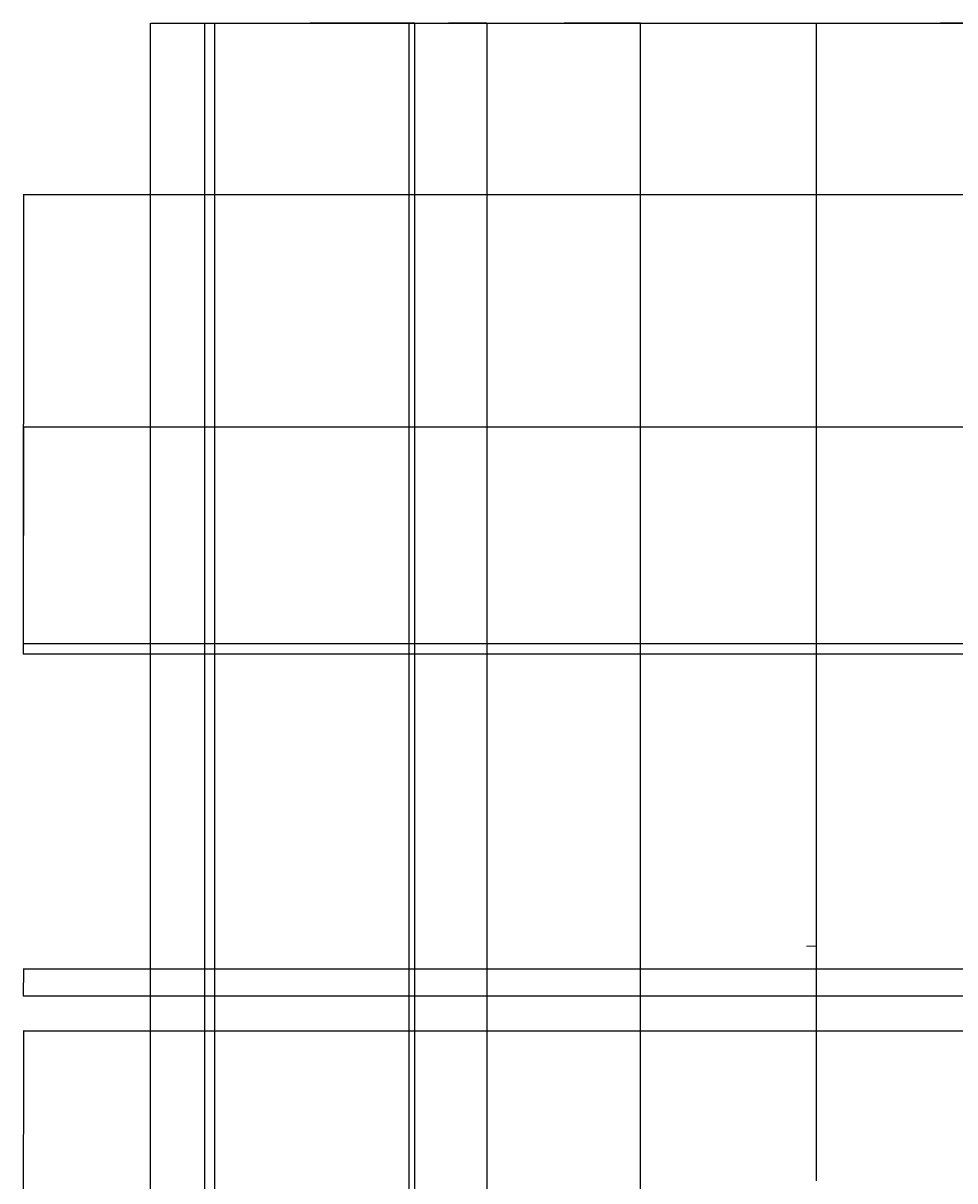
# Model space of a CAD drawing. Units: inches. Extents: x 2029 to 8798, y 1998 to 6373.
# Tile 3 of 11: x 2030 to 2855, y 5347 to 6373. Entities that reach past the tile are written whole.
import ezdxf

# ---------------------------------------------------------------- set-up
doc = ezdxf.new("R2010")
doc.units = ezdxf.units.IN
doc.layers.add('A-ANNO-DIMS', color=2, linetype='Continuous', lineweight=18)
doc.layers.add('A-GENM-REFR', color=8, linetype='Continuous', lineweight=13)
doc.styles.get("Standard").update_dxf_attribs({"font": 'arial.ttf'})
doc.dimstyles.get("Standard").update_dxf_attribs({"dimtxt": 0.18, "dimasz": 0.18, "dimexe": 0.18, "dimexo": 0.0625, "dimgap": 0.09, "dimtad": 0, "dimtih": 1, "dimtoh": 1, "dimdec": 4, "dimzin": 0, "dimdsep": 46, "dimtxsty": 'Standard', "dimcen": 0.09, "dimadec": 0, "dimazin": 0, "dimtfac": 1, "dimtdec": 4, "dimtofl": 0, "dimtmove": 0, "dimatfit": 3, "dimfxl": 1, "dimtolj": 1, "dimtzin": 0, "dimarcsym": 0})

# ---------------------------------------------------------------- blocks, each defined once
blk = doc.blocks.new('*D45')
at = {"layer": 'A-ANNO-DIMS', "color": 0, "lineweight": -2, "transparency": 16777216}
for p, q in [((2199.5, 5019), (2199.5, 6372.5)), ((2199.7, 6372.4), (2285.3, 6372.4)), ((2371.4, 6372.4), (2285.8, 6372.4)), ((2371.5, 5019), (2371.5, 6372.5))]:
    blk.add_line(p, q, dxfattribs=at)
at = {"layer": 'A-ANNO-DIMS', "color": 0, "transparency": 16777216}
for points in [[(2199.7, 6372.4), (2199.7, 6372.3), (2199.5, 6372.4)], [(2371.4, 6372.4), (2371.4, 6372.3), (2371.5, 6372.4)]]:
    blk.add_solid(points, dxfattribs=at)
at = {"layer": 'Defpoints', "color": 0, "transparency": 16777216}
for p in [(2371.5, 6372.4), (2199.5, 5019), (2371.5, 5019)]:
    blk.add_point(p, dxfattribs=at)
at = {"layer": 'A-ANNO-DIMS', "color": 0, "transparency": 16777216, "insert": (2285.5, 6372.4), "char_height": 0.18, "attachment_point": 5}
blk.add_mtext('\\A1;172', dxfattribs=at)
blk = doc.blocks.new('*D46')
at = {"layer": 'A-ANNO-DIMS', "color": 0, "lineweight": -2, "transparency": 16777216}
for p, q in [((2371.5, 5019), (2371.5, 6372.5)), ((2371.7, 6372.4), (2405.8, 6372.4)), ((2440.4, 6372.4), (2406.3, 6372.4)), ((2440.5, 5019), (2440.5, 6372.5))]:
    blk.add_line(p, q, dxfattribs=at)
at = {"layer": 'A-ANNO-DIMS', "color": 0, "transparency": 16777216}
for points in [[(2371.7, 6372.4), (2371.7, 6372.3), (2371.5, 6372.4)], [(2440.4, 6372.4), (2440.4, 6372.3), (2440.5, 6372.4)]]:
    blk.add_solid(points, dxfattribs=at)
at = {"layer": 'Defpoints', "color": 0, "transparency": 16777216}
for p in [(2440.5, 6372.4), (2371.5, 5019), (2440.5, 5019)]:
    blk.add_point(p, dxfattribs=at)
at = {"layer": 'A-ANNO-DIMS', "color": 0, "transparency": 16777216, "insert": (2406, 6372.4), "char_height": 0.18, "attachment_point": 5}
blk.add_mtext('\\A1;69', dxfattribs=at)
blk = doc.blocks.new('*D47')
at = {"layer": 'A-ANNO-DIMS', "color": 0, "lineweight": -2, "transparency": 16777216}
for p, q in [((2440.5, 5019), (2440.5, 6372.5)), ((2440.7, 6372.4), (2508.3, 6372.4)), ((2576.4, 6372.4), (2508.8, 6372.4)), ((2576.5, 5019), (2576.5, 6372.5))]:
    blk.add_line(p, q, dxfattribs=at)
at = {"layer": 'A-ANNO-DIMS', "color": 0, "transparency": 16777216}
for points in [[(2440.7, 6372.4), (2440.7, 6372.3), (2440.5, 6372.4)], [(2576.4, 6372.4), (2576.4, 6372.3), (2576.5, 6372.4)]]:
    blk.add_solid(points, dxfattribs=at)
at = {"layer": 'Defpoints', "color": 0, "transparency": 16777216}
for p in [(2576.5, 6372.4), (2440.5, 5019), (2576.5, 5019)]:
    blk.add_point(p, dxfattribs=at)
at = {"layer": 'A-ANNO-DIMS', "color": 0, "transparency": 16777216, "insert": (2508.5, 6372.4), "char_height": 0.18, "attachment_point": 5}
blk.add_mtext('\\A1;136', dxfattribs=at)
blk = doc.blocks.new('*D49')
at = {"layer": 'A-ANNO-DIMS', "color": 0, "lineweight": -2, "transparency": 16777216}
for p, q in [((2190.5, 4210.1), (2190.5, 6372.5)), ((2190.7, 6372.4), (2283.3, 6372.4)), ((2376.4, 6372.4), (2283.8, 6372.4)), ((2376.5, 4210.1), (2376.5, 6372.5))]:
    blk.add_line(p, q, dxfattribs=at)
at = {"layer": 'A-ANNO-DIMS', "color": 0, "transparency": 16777216}
for points in [[(2190.7, 6372.4), (2190.7, 6372.3), (2190.5, 6372.4)], [(2376.4, 6372.4), (2376.4, 6372.3), (2376.5, 6372.4)]]:
    blk.add_solid(points, dxfattribs=at)
at = {"layer": 'Defpoints', "color": 0, "transparency": 16777216}
for p in [(2376.5, 6372.4), (2190.5, 4210), (2376.5, 4210)]:
    blk.add_point(p, dxfattribs=at)
at = {"layer": 'A-ANNO-DIMS', "color": 0, "transparency": 16777216, "insert": (2283.5, 6372.4), "char_height": 0.18, "attachment_point": 5}
blk.add_mtext('\\A1;186', dxfattribs=at)
blk = doc.blocks.new('*D61')
at = {"layer": 'A-ANNO-DIMS', "color": 0, "lineweight": -2, "transparency": 16777216}
for p, q in [((2732.5, 5347.1), (2732.5, 6372.5)), ((2732.7, 6372.4), (2841.7, 6372.4)), ((2951.3, 6372.4), (2842.3, 6372.4)), ((2951.5, 5347.1), (2951.5, 6372.5))]:
    blk.add_line(p, q, dxfattribs=at)
at = {"layer": 'A-ANNO-DIMS', "color": 0, "transparency": 16777216}
for points in [[(2732.7, 6372.4), (2732.7, 6372.3), (2732.5, 6372.4)], [(2951.3, 6372.4), (2951.3, 6372.3), (2951.5, 6372.4)]]:
    blk.add_solid(points, dxfattribs=at)
at = {"layer": 'Defpoints', "color": 0, "transparency": 16777216}
for p in [(2951.5, 6372.4), (2732.5, 5347), (2951.5, 5347)]:
    blk.add_point(p, dxfattribs=at)
at = {"layer": 'A-ANNO-DIMS', "color": 0, "transparency": 16777216, "insert": (2842, 6372.4), "char_height": 0.18, "attachment_point": 5}
blk.add_mtext('\\A1;219', dxfattribs=at)
blk = doc.blocks.new('*D75')
at = {"layer": 'A-ANNO-DIMS', "color": 0, "lineweight": -2, "transparency": 16777216}
for p, q in [((3887.7, 6220.6), (2029.6, 6220.6)), ((2029.8, 6220.4), (2029.8, 6017.3)), ((2029.8, 5813.8), (2029.8, 6016.9)), ((3887.7, 5813.6), (2029.6, 5813.6))]:
    blk.add_line(p, q, dxfattribs=at)
at = {"layer": 'A-ANNO-DIMS', "color": 0, "transparency": 16777216}
for points in [[(2029.8, 6220.4), (2029.8, 6220.4), (2029.8, 6220.6)], [(2029.8, 5813.8), (2029.8, 5813.8), (2029.8, 5813.6)]]:
    blk.add_solid(points, dxfattribs=at)
at = {"layer": 'Defpoints', "color": 0, "transparency": 16777216}
for p in [(2029.8, 6220.6), (3887.8, 6220.6), (3887.8, 5813.6)]:
    blk.add_point(p, dxfattribs=at)
at = {"layer": 'A-ANNO-DIMS', "color": 0, "transparency": 16777216, "insert": (2029.8, 6017.1), "char_height": 0.18, "attachment_point": 5}
blk.add_mtext('\\A1;407', dxfattribs=at)
blk = doc.blocks.new('*D79')
at = {"layer": 'A-ANNO-DIMS', "color": 0, "lineweight": -2, "transparency": 16777216}
for p, q in [((4043.7, 6014.6), (2029.6, 6014.6)), ((2029.8, 6014.4), (2029.8, 5918.8)), ((2029.8, 5822.8), (2029.8, 5918.4)), ((4043.7, 5822.6), (2029.6, 5822.6))]:
    blk.add_line(p, q, dxfattribs=at)
at = {"layer": 'A-ANNO-DIMS', "color": 0, "transparency": 16777216}
for points in [[(2029.8, 6014.4), (2029.8, 6014.4), (2029.8, 6014.6)], [(2029.8, 5822.8), (2029.8, 5822.8), (2029.8, 5822.6)]]:
    blk.add_solid(points, dxfattribs=at)
at = {"layer": 'Defpoints', "color": 0, "transparency": 16777216}
for p in [(2029.8, 6014.6), (4043.8, 6014.6), (4043.8, 5822.6)]:
    blk.add_point(p, dxfattribs=at)
at = {"layer": 'A-ANNO-DIMS', "color": 0, "transparency": 16777216, "insert": (2029.8, 5918.6), "char_height": 0.18, "attachment_point": 5}
blk.add_mtext('\\A1;192', dxfattribs=at)
blk = doc.blocks.new('*D88')
at = {"layer": 'A-ANNO-DIMS', "color": 0, "lineweight": -2, "transparency": 16777216}
for p, q in [((2142.5, 4445.1), (2142.5, 6372.5)), ((2142.7, 6372.4), (3266.2, 6372.4)), ((4390.6, 6372.4), (3267.1, 6372.4)), ((4390.8, 4574.1), (4390.8, 6372.5))]:
    blk.add_line(p, q, dxfattribs=at)
at = {"layer": 'A-ANNO-DIMS', "color": 0, "transparency": 16777216}
for points in [[(2142.7, 6372.4), (2142.7, 6372.3), (2142.5, 6372.4)], [(4390.6, 6372.4), (4390.6, 6372.3), (4390.8, 6372.4)]]:
    blk.add_solid(points, dxfattribs=at)
at = {"layer": 'Defpoints', "color": 0, "transparency": 16777216}
for p in [(4390.8, 6372.4), (4390.8, 4574), (2142.5, 4445)]:
    blk.add_point(p, dxfattribs=at)
at = {"layer": 'A-ANNO-DIMS', "color": 0, "transparency": 16777216, "insert": (3266.7, 6372.4), "char_height": 0.18, "attachment_point": 5}
blk.add_mtext('\\A1;2248.2', dxfattribs=at)
blk = doc.blocks.new('*D105')
at = {"layer": 'A-ANNO-DIMS', "color": 0, "lineweight": -2, "transparency": 16777216}
for p, q in [((3968.7, 5479.6), (2029.6, 5479.6)), ((2029.8, 5479.4), (2029.8, 5388.3)), ((2029.8, 5296.8), (2029.8, 5387.9)), ((3968.7, 5296.6), (2029.6, 5296.6))]:
    blk.add_line(p, q, dxfattribs=at)
at = {"layer": 'A-ANNO-DIMS', "color": 0, "transparency": 16777216}
for points in [[(2029.8, 5479.4), (2029.8, 5479.4), (2029.8, 5479.6)], [(2029.8, 5296.8), (2029.8, 5296.8), (2029.8, 5296.6)]]:
    blk.add_solid(points, dxfattribs=at)
at = {"layer": 'Defpoints', "color": 0, "transparency": 16777216}
for p in [(2029.8, 5479.6), (3968.8, 5479.6), (3968.8, 5296.6)]:
    blk.add_point(p, dxfattribs=at)
at = {"layer": 'A-ANNO-DIMS', "color": 0, "transparency": 16777216, "insert": (2029.8, 5388.1), "char_height": 0.18, "attachment_point": 5}
blk.add_mtext('\\A1;183', dxfattribs=at)
blk = doc.blocks.new('*D108')
at = {"layer": 'A-ANNO-DIMS', "color": 0, "lineweight": -2, "transparency": 16777216}
for p, q in [((4256.3, 5534.6), (2029.6, 5534.6)), ((2029.8, 5534.4), (2029.8, 5522.8)), ((2029.8, 5510.8), (2029.8, 5522.4)), ((4256.3, 5510.6), (2029.6, 5510.6))]:
    blk.add_line(p, q, dxfattribs=at)
at = {"layer": 'A-ANNO-DIMS', "color": 0, "transparency": 16777216}
for points in [[(2029.8, 5534.4), (2029.8, 5534.4), (2029.8, 5534.6)], [(2029.8, 5510.8), (2029.8, 5510.8), (2029.8, 5510.6)]]:
    blk.add_solid(points, dxfattribs=at)
at = {"layer": 'Defpoints', "color": 0, "transparency": 16777216}
for p in [(4256.4, 5534.6), (2029.8, 5510.6), (4256.4, 5510.6)]:
    blk.add_point(p, dxfattribs=at)
at = {"layer": 'A-ANNO-DIMS', "color": 0, "transparency": 16777216, "insert": (2029.8, 5522.6), "char_height": 0.18, "attachment_point": 5}
blk.add_mtext('\\A1;24', dxfattribs=at)

msp = doc.modelspace()

# ---------------------------------------------------------------- linework, layer by layer
at = {"layer": 'A-GENM-REFR'}
msp.add_line((2723.5398, 5554.822), (2732.5398, 5554.822), dxfattribs=at)

# ---------------------------------------------------------------- dimensions: what is measured, and where the dimension line sits
at = {"layer": 'A-ANNO-DIMS'}
for base, p1, p2, override, picture, middle in [((4390.7657, 6372.3623), (2142.5398, 4444.9886), (4390.7657, 4573.9886), {"dimdec": 1, "dimlfac": 1, "dimrnd": 0, "dimzin": 0, "dimdsep": 46, "dimlunit": 2}, '*D88', (3266.6528, 6372.3623)), ((2376.5398, 6372.3623), (2190.5398, 4209.9886), (2376.5398, 4209.9886), {"dimdec": 0, "dimlfac": 1, "dimrnd": 0, "dimzin": 0, "dimdsep": 46, "dimlunit": 2}, '*D49', (2283.5398, 6372.3623)), ((2371.5398, 6372.3623), (2199.5398, 5018.9585), (2371.5398, 5018.9585), {"dimdec": 0, "dimlfac": 1, "dimrnd": 0, "dimzin": 0, "dimdsep": 46, "dimlunit": 2}, '*D45', (2285.5398, 6372.3623)), ((2440.5398, 6372.3623), (2371.5398, 5018.9585), (2440.5398, 5018.9585), {"dimdec": 0, "dimlfac": 1, "dimrnd": 0, "dimzin": 0, "dimdsep": 46, "dimlunit": 2}, '*D46', (2406.0398, 6372.3623)), ((2576.5398, 6372.3623), (2440.5398, 5018.9585), (2576.5398, 5018.9585), {"dimdec": 0, "dimlfac": 1, "dimrnd": 0, "dimzin": 0, "dimdsep": 46, "dimlunit": 2}, '*D47', (2508.5398, 6372.3623)), ((2951.5292, 6372.3623), (2732.5398, 5346.9886), (2951.5292, 5346.9886), {"dimdec": 0, "dimlfac": 1, "dimrnd": 0, "dimzin": 0, "dimdsep": 46, "dimlunit": 2}, '*D61', (2842.0345, 6372.3623))]:
    dim = msp.add_linear_dim(base=base, p1=p1, p2=p2, dimstyle='Standard', override=override, dxfattribs=at)
    dim.commit()
    dim.dimension.update_dxf_attribs({"geometry": picture, "text_midpoint": middle})
for base, p1, p2, picture, middle in [((2029.7898, 6220.6123), (3887.7657, 5813.6123), (3887.7657, 6220.6123), '*D75', (2029.7898, 6017.1123)), ((2029.7898, 6014.6123), (4043.7657, 5822.6123), (4043.7657, 6014.6123), '*D79', (2029.7898, 5918.6123)), ((2029.7898, 5510.6123), (4256.3869, 5534.6123), (4256.3869, 5510.6123), '*D108', (2029.7898, 5522.6123)), ((2029.7898, 5479.6123), (3968.7657, 5296.6123), (3968.7657, 5479.6123), '*D105', (2029.7898, 5388.1123))]:
    dim = msp.add_linear_dim(base=base, p1=p1, p2=p2, angle=90, dimstyle='Standard', override={"dimdec": 0, "dimlfac": 1, "dimrnd": 0, "dimzin": 0, "dimdsep": 46, "dimlunit": 2}, dxfattribs=at)
    dim.commit()
    dim.dimension.update_dxf_attribs({"geometry": picture, "text_midpoint": middle})

doc.saveas('drawing.dxf')
